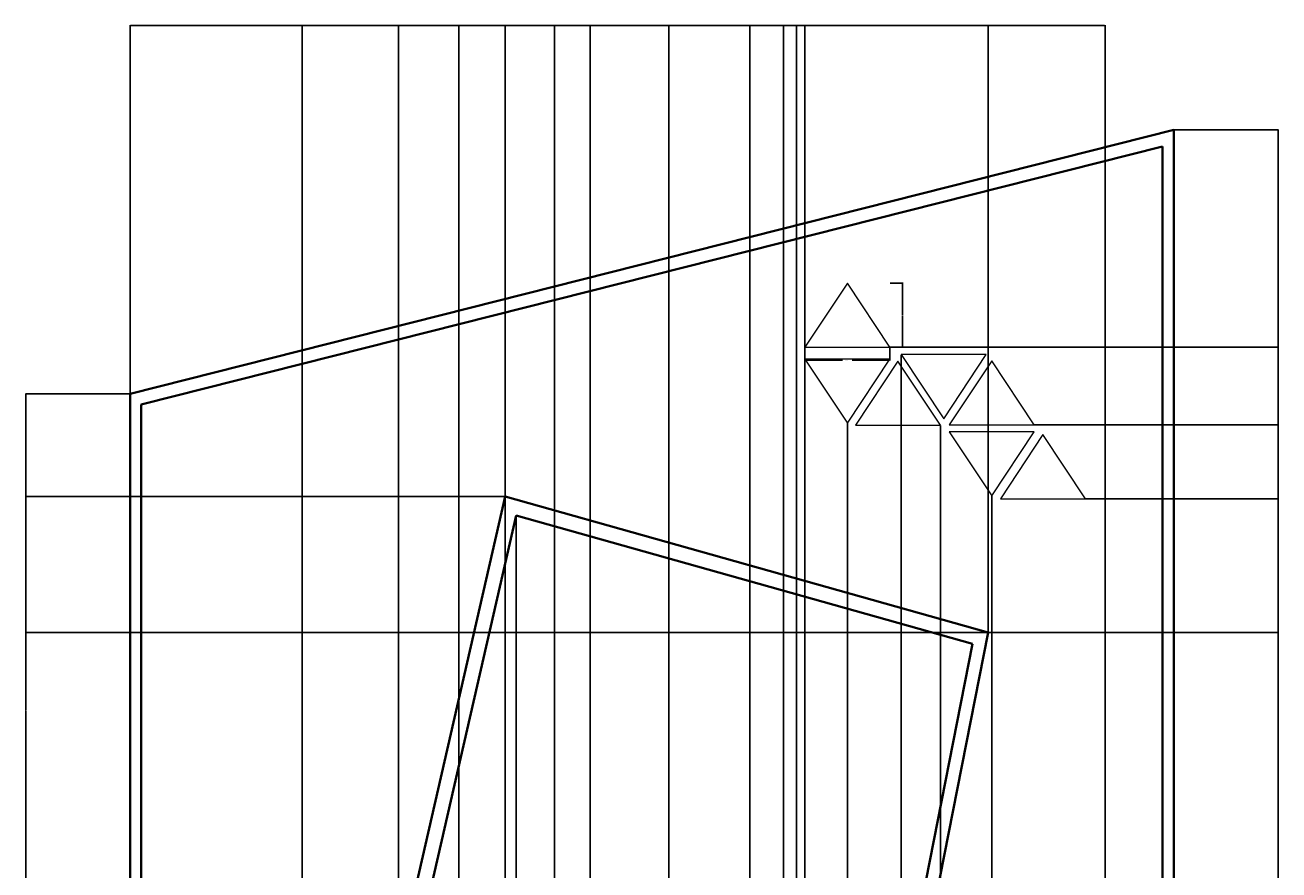
# Model space of a CAD drawing. Units: feet. Extents: x 2373 to 3800, y 799 to 1842.
# Tile 4 of 4: x 3224 to 3800, y 1453 to 1842. Entities that reach past the tile are written whole.
import ezdxf

# ---------------------------------------------------------------- set-up
doc = ezdxf.new("R2010")
doc.units = ezdxf.units.FT
for name, color, linetype, lineweight in [('A-ANNO-DIMS', 2, 'Continuous', 18), ('A-ELEV', 7, 'Continuous', 35), ('E-LITE', 2, 'Continuous', 18)]:
    doc.layers.add(name, color=color, linetype=linetype, lineweight=lineweight)
doc.styles.get("Standard").update_dxf_attribs({"font": 'arial.ttf'})
doc.dimstyles.get("Standard").update_dxf_attribs({"dimtxt": 0.18, "dimasz": 0.18, "dimexe": 0.18, "dimexo": 0.0625, "dimgap": 0.09, "dimtad": 0, "dimtih": 1, "dimtoh": 1, "dimdec": 1, "dimzin": 0, "dimdsep": 46, "dimlunit": 3, "dimtxsty": 'Standard', "dimcen": 0.09, "dimadec": 0, "dimazin": 0, "dimtfac": 1, "dimtdec": 1, "dimtofl": 0, "dimtmove": 0, "dimatfit": 3, "dimfxl": 1, "dimtolj": 1, "dimtzin": 0, "dimarcsym": 0})

# ---------------------------------------------------------------- blocks, each defined once
blk = doc.blocks.new('LIGHT-TRIANGLE')
blk.add_lwpolyline([(2765.64, 1685.95), (2746.09, 1715.45), (2726.54, 1685.95)], close=True)
blk = doc.blocks.new('*D2')
at = {"layer": 'A-ANNO-DIMS', "color": 0, "lineweight": -2, "transparency": 16777216}
for p, q in [((3582.33, 1693.47), (3582.33, 1687.49)), ((3621.43, 1693.47), (3621.43, 1687.49)), ((3582.51, 1687.67), (3599.66, 1687.67)), ((3621.25, 1687.67), (3604.1, 1687.67))]:
    blk.add_line(p, q, dxfattribs=at)
at = {"layer": 'A-ANNO-DIMS', "color": 0, "transparency": 16777216}
for points in [[(3582.51, 1687.7), (3582.51, 1687.64), (3582.33, 1687.67)], [(3621.25, 1687.7), (3621.25, 1687.64), (3621.43, 1687.67)]]:
    blk.add_solid(points, dxfattribs=at)
at = {"layer": 'Defpoints', "color": 0, "transparency": 16777216}
for p in [(3582.33, 1693.53), (3621.43, 1693.53), (3621.43, 1687.67)]:
    blk.add_point(p, dxfattribs=at)
at = {"layer": 'A-ANNO-DIMS', "color": 0, "transparency": 16777216, "insert": (3601.88, 1687.67), "char_height": 0.18, "attachment_point": 5}
blk.add_mtext('\\A1;TRIANGLE FEATURE LIGHT 39 TYP.', dxfattribs=at)
blk = doc.blocks.new('*D3')
at = {"layer": 'A-ANNO-DIMS', "color": 0, "lineweight": -2, "transparency": 16777216}
for p, q in [((3621.5, 1723.04), (3627.48, 1723.04)), ((3627.3, 1722.86), (3627.3, 1708.47)), ((3627.3, 1693.71), (3627.3, 1708.1)), ((3621.5, 1693.53), (3627.48, 1693.53))]:
    blk.add_line(p, q, dxfattribs=at)
at = {"layer": 'A-ANNO-DIMS', "color": 0, "transparency": 16777216}
for points in [[(3627.27, 1722.86), (3627.33, 1722.86), (3627.3, 1723.04)], [(3627.27, 1693.71), (3627.33, 1693.71), (3627.3, 1693.53)]]:
    blk.add_solid(points, dxfattribs=at)
at = {"layer": 'Defpoints', "color": 0, "transparency": 16777216}
for p in [(3621.43, 1723.04), (3627.3, 1723.04), (3621.43, 1693.53)]:
    blk.add_point(p, dxfattribs=at)
at = {"layer": 'A-ANNO-DIMS', "color": 0, "transparency": 16777216, "insert": (3627.3, 1708.28), "char_height": 0.18, "attachment_point": 5}
blk.add_mtext('\\A1;30 TYP.', dxfattribs=at)
blk = doc.blocks.new('*D8')
at = {"layer": 'A-ANNO-DIMS', "color": 0, "lineweight": -2, "transparency": 16777216}
for p, q in [((3752.05, 1793.54), (3800.17, 1793.54)), ((3799.99, 1793.36), (3799.99, 1320.78)), ((3799.99, 847.83), (3799.99, 1320.41)), ((3752.05, 847.65), (3800.17, 847.65))]:
    blk.add_line(p, q, dxfattribs=at)
at = {"layer": 'A-ANNO-DIMS', "color": 0, "transparency": 16777216}
for points in [[(3799.96, 1793.36), (3800.02, 1793.36), (3799.99, 1793.54)], [(3799.96, 847.83), (3800.02, 847.83), (3799.99, 847.65)]]:
    blk.add_solid(points, dxfattribs=at)
at = {"layer": 'Defpoints', "color": 0, "transparency": 16777216}
for p in [(3751.99, 1793.54), (3799.99, 1793.54), (3751.99, 847.65)]:
    blk.add_point(p, dxfattribs=at)
at = {"layer": 'A-ANNO-DIMS', "color": 0, "transparency": 16777216, "insert": (3799.99, 1320.6), "char_height": 0.18, "attachment_point": 5}
blk.add_mtext('\\A1;945.9', dxfattribs=at)
blk = doc.blocks.new('*D12')
at = {"layer": 'A-ANNO-DIMS', "color": 0, "lineweight": -2, "transparency": 16777216}
for p, q in [((3271.92, 1672.17), (3223.81, 1672.17)), ((3223.99, 1671.99), (3223.99, 1526.69)), ((3223.99, 1381.03), (3223.99, 1526.33)), ((3271.92, 1380.85), (3223.81, 1380.85))]:
    blk.add_line(p, q, dxfattribs=at)
at = {"layer": 'A-ANNO-DIMS', "color": 0, "transparency": 16777216}
for points in [[(3223.96, 1671.99), (3224.02, 1671.99), (3223.99, 1672.17)], [(3223.96, 1381.03), (3224.02, 1381.03), (3223.99, 1380.85)]]:
    blk.add_solid(points, dxfattribs=at)
at = {"layer": 'Defpoints', "color": 0, "transparency": 16777216}
for p in [(3223.99, 1672.17), (3271.99, 1672.17), (3271.99, 1380.85)]:
    blk.add_point(p, dxfattribs=at)
at = {"layer": 'A-ANNO-DIMS', "color": 0, "transparency": 16777216, "insert": (3223.99, 1526.51), "char_height": 0.18, "attachment_point": 5}
blk.add_mtext('\\A1;291.3', dxfattribs=at)
blk = doc.blocks.new('*D13')
at = {"layer": 'A-ANNO-DIMS', "color": 0, "lineweight": -2, "transparency": 16777216}
for p, q in [((3271.99, 1380.91), (3271.99, 1841.72)), ((3272.17, 1841.54), (3347.21, 1841.54)), ((3423.01, 1841.54), (3347.97, 1841.54)), ((3423.19, 1380.91), (3423.19, 1841.72))]:
    blk.add_line(p, q, dxfattribs=at)
at = {"layer": 'A-ANNO-DIMS', "color": 0, "transparency": 16777216}
for points in [[(3272.17, 1841.57), (3272.17, 1841.51), (3271.99, 1841.54)], [(3423.01, 1841.57), (3423.01, 1841.51), (3423.19, 1841.54)]]:
    blk.add_solid(points, dxfattribs=at)
at = {"layer": 'Defpoints', "color": 0, "transparency": 16777216}
for p in [(3423.19, 1841.54), (3271.99, 1380.85), (3423.19, 1380.85)]:
    blk.add_point(p, dxfattribs=at)
at = {"layer": 'A-ANNO-DIMS', "color": 0, "transparency": 16777216, "insert": (3347.59, 1841.54), "char_height": 0.18, "attachment_point": 5}
blk.add_mtext('\\A1;151.2', dxfattribs=at)
blk = doc.blocks.new('*D14')
at = {"layer": 'A-ANNO-DIMS', "color": 0, "lineweight": -2, "transparency": 16777216}
for p, q in [((3423.19, 1145.85), (3423.19, 1841.72)), ((3423.37, 1841.54), (3471.07, 1841.54)), ((3519.56, 1841.54), (3471.86, 1841.54)), ((3519.74, 1442.83), (3519.74, 1841.72))]:
    blk.add_line(p, q, dxfattribs=at)
at = {"layer": 'A-ANNO-DIMS', "color": 0, "transparency": 16777216}
for points in [[(3423.37, 1841.57), (3423.37, 1841.51), (3423.19, 1841.54)], [(3519.56, 1841.57), (3519.56, 1841.51), (3519.74, 1841.54)]]:
    blk.add_solid(points, dxfattribs=at)
at = {"layer": 'Defpoints', "color": 0, "transparency": 16777216}
for p in [(3519.74, 1841.54), (3519.74, 1442.77), (3423.19, 1145.79)]:
    blk.add_point(p, dxfattribs=at)
at = {"layer": 'A-ANNO-DIMS', "color": 0, "transparency": 16777216, "insert": (3471.46, 1841.54), "char_height": 0.18, "attachment_point": 5}
blk.add_mtext('\\A1;96.54', dxfattribs=at)
blk = doc.blocks.new('*D16')
at = {"layer": 'A-ANNO-DIMS', "color": 0, "lineweight": -2, "transparency": 16777216}
for p, q in [((3444.52, 1624.94), (3444.52, 1841.72)), ((3444.7, 1841.54), (3555.12, 1841.54)), ((3666.48, 1841.54), (3556.05, 1841.54)), ((3666.66, 1562.48), (3666.66, 1841.72))]:
    blk.add_line(p, q, dxfattribs=at)
at = {"layer": 'A-ANNO-DIMS', "color": 0, "transparency": 16777216}
for points in [[(3444.7, 1841.57), (3444.7, 1841.51), (3444.52, 1841.54)], [(3666.48, 1841.57), (3666.48, 1841.51), (3666.66, 1841.54)]]:
    blk.add_solid(points, dxfattribs=at)
at = {"layer": 'Defpoints', "color": 0, "transparency": 16777216}
for p in [(3666.66, 1841.54), (3444.52, 1624.88), (3666.66, 1562.42)]:
    blk.add_point(p, dxfattribs=at)
at = {"layer": 'A-ANNO-DIMS', "color": 0, "transparency": 16777216, "insert": (3555.59, 1841.54), "char_height": 0.18, "attachment_point": 5}
blk.add_mtext('\\A1;222.14', dxfattribs=at)
blk = doc.blocks.new('*D17')
at = {"layer": 'A-ANNO-DIMS', "color": 0, "lineweight": -2, "transparency": 16777216}
for p, q in [((3666.72, 1562.42), (3800.17, 1562.42)), ((3799.99, 1562.24), (3799.99, 1354.28)), ((3799.99, 1145.97), (3799.99, 1353.92)), ((3578.6, 1145.79), (3800.17, 1145.79))]:
    blk.add_line(p, q, dxfattribs=at)
at = {"layer": 'A-ANNO-DIMS', "color": 0, "transparency": 16777216}
for points in [[(3799.96, 1562.24), (3800.02, 1562.24), (3799.99, 1562.42)], [(3799.96, 1145.97), (3800.02, 1145.97), (3799.99, 1145.79)]]:
    blk.add_solid(points, dxfattribs=at)
at = {"layer": 'Defpoints', "color": 0, "transparency": 16777216}
for p in [(3666.66, 1562.42), (3799.99, 1562.42), (3578.54, 1145.79)]:
    blk.add_point(p, dxfattribs=at)
at = {"layer": 'A-ANNO-DIMS', "color": 0, "transparency": 16777216, "insert": (3799.99, 1354.1), "char_height": 0.18, "attachment_point": 5}
blk.add_mtext('\\A1;416.6', dxfattribs=at)
blk = doc.blocks.new('*D20')
at = {"layer": 'A-ANNO-DIMS', "color": 0, "lineweight": -2, "transparency": 16777216}
for p, q in [((3572.43, 945.53), (3572.43, 1841.72)), ((3572.61, 1841.54), (3645.95, 1841.54)), ((3720.2, 1841.54), (3646.87, 1841.54)), ((3720.38, 1113.42), (3720.38, 1841.72))]:
    blk.add_line(p, q, dxfattribs=at)
at = {"layer": 'A-ANNO-DIMS', "color": 0, "transparency": 16777216}
for points in [[(3572.61, 1841.57), (3572.61, 1841.51), (3572.43, 1841.54)], [(3720.2, 1841.57), (3720.2, 1841.51), (3720.38, 1841.54)]]:
    blk.add_solid(points, dxfattribs=at)
at = {"layer": 'Defpoints', "color": 0, "transparency": 16777216}
for p in [(3720.38, 1841.54), (3720.38, 1113.36), (3572.43, 945.46)]:
    blk.add_point(p, dxfattribs=at)
at = {"layer": 'A-ANNO-DIMS', "color": 0, "transparency": 16777216, "insert": (3646.41, 1841.54), "char_height": 0.18, "attachment_point": 5}
blk.add_mtext('\\A1;147.95', dxfattribs=at)
blk = doc.blocks.new('*D23')
at = {"layer": 'A-ANNO-DIMS', "color": 0, "lineweight": -2, "transparency": 16777216}
for p, q in [((3483.65, 925.75), (3483.65, 1841.72)), ((3483.83, 1841.54), (3519.95, 1841.54)), ((3556.84, 1841.54), (3520.73, 1841.54)), ((3557.02, 1097.65), (3557.02, 1841.72))]:
    blk.add_line(p, q, dxfattribs=at)
at = {"layer": 'A-ANNO-DIMS', "color": 0, "transparency": 16777216}
for points in [[(3483.83, 1841.57), (3483.83, 1841.51), (3483.65, 1841.54)], [(3556.84, 1841.57), (3556.84, 1841.51), (3557.02, 1841.54)]]:
    blk.add_solid(points, dxfattribs=at)
at = {"layer": 'Defpoints', "color": 0, "transparency": 16777216}
for p in [(3557.02, 1841.54), (3557.02, 1097.59), (3483.65, 925.69)]:
    blk.add_point(p, dxfattribs=at)
at = {"layer": 'A-ANNO-DIMS', "color": 0, "transparency": 16777216, "insert": (3520.34, 1841.54), "char_height": 0.18, "attachment_point": 5}
blk.add_mtext('\\A1;73.37', dxfattribs=at)
blk = doc.blocks.new('*D25')
at = {"layer": 'A-ANNO-DIMS', "color": 0, "lineweight": -2, "transparency": 16777216}
for p, q in [((3271.99, 1672.23), (3271.99, 1841.72)), ((3272.17, 1841.54), (3357.8, 1841.54)), ((3444.34, 1841.54), (3358.71, 1841.54)), ((3444.52, 1624.94), (3444.52, 1841.72))]:
    blk.add_line(p, q, dxfattribs=at)
at = {"layer": 'A-ANNO-DIMS', "color": 0, "transparency": 16777216}
for points in [[(3272.17, 1841.57), (3272.17, 1841.51), (3271.99, 1841.54)], [(3444.34, 1841.57), (3444.34, 1841.51), (3444.52, 1841.54)]]:
    blk.add_solid(points, dxfattribs=at)
at = {"layer": 'Defpoints', "color": 0, "transparency": 16777216}
for p in [(3444.52, 1841.54), (3271.99, 1672.17), (3444.52, 1624.88)]:
    blk.add_point(p, dxfattribs=at)
at = {"layer": 'A-ANNO-DIMS', "color": 0, "transparency": 16777216, "insert": (3358.25, 1841.54), "char_height": 0.18, "attachment_point": 5}
blk.add_mtext('\\A1;172.53', dxfattribs=at)
blk = doc.blocks.new('*D26')
at = {"layer": 'A-ANNO-DIMS', "color": 0, "lineweight": -2, "transparency": 16777216}
for p, q in [((3444.46, 1624.88), (3223.81, 1624.88)), ((3223.99, 1624.7), (3223.99, 1593.83)), ((3223.99, 1562.6), (3223.99, 1593.47)), ((3666.6, 1562.42), (3223.81, 1562.42))]:
    blk.add_line(p, q, dxfattribs=at)
at = {"layer": 'A-ANNO-DIMS', "color": 0, "transparency": 16777216}
for points in [[(3223.96, 1624.7), (3224.02, 1624.7), (3223.99, 1624.88)], [(3223.96, 1562.6), (3224.02, 1562.6), (3223.99, 1562.42)]]:
    blk.add_solid(points, dxfattribs=at)
at = {"layer": 'Defpoints', "color": 0, "transparency": 16777216}
for p in [(3444.52, 1624.88), (3223.99, 1562.42), (3666.66, 1562.42)]:
    blk.add_point(p, dxfattribs=at)
at = {"layer": 'A-ANNO-DIMS', "color": 0, "transparency": 16777216, "insert": (3223.99, 1593.65), "char_height": 0.18, "attachment_point": 5}
blk.add_mtext('\\A1;62.46', dxfattribs=at)
blk = doc.blocks.new('*D27')
at = {"layer": 'A-ANNO-DIMS', "color": 0, "lineweight": -2, "transparency": 16777216}
for p, q in [((3444.52, 1624.82), (3444.52, 799.47)), ((3449.58, 1616.05), (3449.58, 799.47)), ((3444.7, 799.65), (3446.65, 799.65)), ((3449.4, 799.65), (3447.44, 799.65))]:
    blk.add_line(p, q, dxfattribs=at)
at = {"layer": 'A-ANNO-DIMS', "color": 0, "transparency": 16777216}
for points in [[(3444.7, 799.68), (3444.7, 799.62), (3444.52, 799.65)], [(3449.4, 799.68), (3449.4, 799.62), (3449.58, 799.65)]]:
    blk.add_solid(points, dxfattribs=at)
at = {"layer": 'Defpoints', "color": 0, "transparency": 16777216}
for p in [(3444.52, 1624.88), (3449.58, 1616.11), (3449.58, 799.65)]:
    blk.add_point(p, dxfattribs=at)
at = {"layer": 'A-ANNO-DIMS', "color": 0, "transparency": 16777216, "insert": (3447.05, 799.65), "char_height": 0.18, "attachment_point": 5}
blk.add_mtext('\\A1;5.057', dxfattribs=at)
blk = doc.blocks.new('*D29')
at = {"layer": 'A-ANNO-DIMS', "color": 0, "lineweight": -2, "transparency": 16777216}
for p, q in [((3519.74, 1145.85), (3519.74, 1841.72)), ((3519.92, 1841.54), (3548.81, 1841.54)), ((3578.36, 1841.54), (3549.46, 1841.54)), ((3578.54, 1145.85), (3578.54, 1841.72))]:
    blk.add_line(p, q, dxfattribs=at)
at = {"layer": 'A-ANNO-DIMS', "color": 0, "transparency": 16777216}
for points in [[(3519.92, 1841.57), (3519.92, 1841.51), (3519.74, 1841.54)], [(3578.36, 1841.57), (3578.36, 1841.51), (3578.54, 1841.54)]]:
    blk.add_solid(points, dxfattribs=at)
at = {"layer": 'Defpoints', "color": 0, "transparency": 16777216}
for p in [(3578.54, 1841.54), (3519.74, 1145.79), (3578.54, 1145.79)]:
    blk.add_point(p, dxfattribs=at)
at = {"layer": 'A-ANNO-DIMS', "color": 0, "transparency": 16777216, "insert": (3549.14, 1841.54), "char_height": 0.18, "attachment_point": 5}
blk.add_mtext('\\A1;58.8', dxfattribs=at)
blk = doc.blocks.new('*D36')
at = {"layer": 'A-ANNO-DIMS', "color": 0, "lineweight": -2, "transparency": 16777216}
for p, q in [((3351.18, 1010.48), (3351.18, 1841.72)), ((3351.36, 1841.54), (3372.95, 1841.54)), ((3395.3, 1841.54), (3373.71, 1841.54)), ((3395.48, 1010.48), (3395.48, 1841.72))]:
    blk.add_line(p, q, dxfattribs=at)
at = {"layer": 'A-ANNO-DIMS', "color": 0, "transparency": 16777216}
for points in [[(3351.36, 1841.57), (3351.36, 1841.51), (3351.18, 1841.54)], [(3395.3, 1841.57), (3395.3, 1841.51), (3395.48, 1841.54)]]:
    blk.add_solid(points, dxfattribs=at)
at = {"layer": 'Defpoints', "color": 0, "transparency": 16777216}
for p in [(3395.48, 1841.54), (3351.18, 1010.41), (3395.48, 1010.41)]:
    blk.add_point(p, dxfattribs=at)
at = {"layer": 'A-ANNO-DIMS', "color": 0, "transparency": 16777216, "insert": (3373.33, 1841.54), "char_height": 0.18, "attachment_point": 5}
blk.add_mtext('\\A1;44.31', dxfattribs=at)
blk = doc.blocks.new('*D37')
at = {"layer": 'A-ANNO-DIMS', "color": 0, "lineweight": -2, "transparency": 16777216}
for p, q in [((3395.48, 1097.65), (3395.48, 1841.72)), ((3395.66, 1841.54), (3430.91, 1841.54)), ((3466.94, 1841.54), (3431.69, 1841.54)), ((3467.12, 1097.65), (3467.12, 1841.72))]:
    blk.add_line(p, q, dxfattribs=at)
at = {"layer": 'A-ANNO-DIMS', "color": 0, "transparency": 16777216}
for points in [[(3395.66, 1841.57), (3395.66, 1841.51), (3395.48, 1841.54)], [(3466.94, 1841.57), (3466.94, 1841.51), (3467.12, 1841.54)]]:
    blk.add_solid(points, dxfattribs=at)
at = {"layer": 'Defpoints', "color": 0, "transparency": 16777216}
for p in [(3467.12, 1841.54), (3395.48, 1097.59), (3467.12, 1097.59)]:
    blk.add_point(p, dxfattribs=at)
at = {"layer": 'A-ANNO-DIMS', "color": 0, "transparency": 16777216, "insert": (3431.3, 1841.54), "char_height": 0.18, "attachment_point": 5}
blk.add_mtext('\\A1;71.63', dxfattribs=at)
blk = doc.blocks.new('*D38')
at = {"layer": 'A-ANNO-DIMS', "color": 0, "lineweight": -2, "transparency": 16777216}
for p, q in [((3467.12, 1097.65), (3467.12, 1841.72)), ((3467.3, 1841.54), (3474.93, 1841.54)), ((3483.47, 1841.54), (3475.84, 1841.54)), ((3483.65, 1097.65), (3483.65, 1841.72))]:
    blk.add_line(p, q, dxfattribs=at)
at = {"layer": 'A-ANNO-DIMS', "color": 0, "transparency": 16777216}
for points in [[(3467.3, 1841.57), (3467.3, 1841.51), (3467.12, 1841.54)], [(3483.47, 1841.57), (3483.47, 1841.51), (3483.65, 1841.54)]]:
    blk.add_solid(points, dxfattribs=at)
at = {"layer": 'Defpoints', "color": 0, "transparency": 16777216}
for p in [(3483.65, 1841.54), (3467.12, 1097.59), (3483.65, 1097.59)]:
    blk.add_point(p, dxfattribs=at)
at = {"layer": 'A-ANNO-DIMS', "color": 0, "transparency": 16777216, "insert": (3475.39, 1841.54), "char_height": 0.18, "attachment_point": 5}
blk.add_mtext('\\A1;16.537', dxfattribs=at)
blk = doc.blocks.new('*D47')
at = {"layer": 'A-ANNO-DIMS', "color": 0, "lineweight": -2, "transparency": 16777216}
for p, q in [((3271.99, 1672.23), (3271.99, 1841.72)), ((3272.17, 1841.54), (3426.7, 1841.54)), ((3582.15, 1841.54), (3427.62, 1841.54)), ((3582.33, 1693.6), (3582.33, 1841.72))]:
    blk.add_line(p, q, dxfattribs=at)
at = {"layer": 'A-ANNO-DIMS', "color": 0, "transparency": 16777216}
for points in [[(3272.17, 1841.57), (3272.17, 1841.51), (3271.99, 1841.54)], [(3582.15, 1841.57), (3582.15, 1841.51), (3582.33, 1841.54)]]:
    blk.add_solid(points, dxfattribs=at)
at = {"layer": 'Defpoints', "color": 0, "transparency": 16777216}
for p in [(3582.33, 1841.54), (3582.33, 1693.53), (3271.99, 1672.17)]:
    blk.add_point(p, dxfattribs=at)
at = {"layer": 'A-ANNO-DIMS', "color": 0, "transparency": 16777216, "insert": (3427.16, 1841.54), "char_height": 0.18, "attachment_point": 5}
blk.add_mtext('\\A1;310.35', dxfattribs=at)
blk = doc.blocks.new('*D48')
at = {"layer": 'A-ANNO-DIMS', "color": 0, "lineweight": -2, "transparency": 16777216}
for p, q in [((3582.33, 1693.47), (3582.33, 799.47)), ((3601.88, 1658.52), (3601.88, 799.47)), ((3582.51, 799.65), (3591.72, 799.65)), ((3601.7, 799.65), (3592.49, 799.65))]:
    blk.add_line(p, q, dxfattribs=at)
at = {"layer": 'A-ANNO-DIMS', "color": 0, "transparency": 16777216}
for points in [[(3582.51, 799.68), (3582.51, 799.62), (3582.33, 799.65)], [(3601.7, 799.68), (3601.7, 799.62), (3601.88, 799.65)]]:
    blk.add_solid(points, dxfattribs=at)
at = {"layer": 'Defpoints', "color": 0, "transparency": 16777216}
for p in [(3582.33, 1693.53), (3601.88, 1658.58), (3601.88, 799.65)]:
    blk.add_point(p, dxfattribs=at)
at = {"layer": 'A-ANNO-DIMS', "color": 0, "transparency": 16777216, "insert": (3592.11, 799.65), "char_height": 0.18, "attachment_point": 5}
blk.add_mtext('\\A1;19.55', dxfattribs=at)
blk = doc.blocks.new('*D49')
at = {"layer": 'A-ANNO-DIMS', "color": 0, "lineweight": -2, "transparency": 16777216}
for p, q in [((3626.67, 1690.12), (3626.67, 799.47)), ((3601.88, 1658.52), (3601.88, 799.47)), ((3602.06, 799.65), (3613.88, 799.65)), ((3626.49, 799.65), (3614.67, 799.65))]:
    blk.add_line(p, q, dxfattribs=at)
at = {"layer": 'A-ANNO-DIMS', "color": 0, "transparency": 16777216}
for points in [[(3602.06, 799.68), (3602.06, 799.62), (3601.88, 799.65)], [(3626.49, 799.68), (3626.49, 799.62), (3626.67, 799.65)]]:
    blk.add_solid(points, dxfattribs=at)
at = {"layer": 'Defpoints', "color": 0, "transparency": 16777216}
for p in [(3626.67, 1690.18), (3601.88, 1658.58), (3626.67, 799.65)]:
    blk.add_point(p, dxfattribs=at)
at = {"layer": 'A-ANNO-DIMS', "color": 0, "transparency": 16777216, "insert": (3614.28, 799.65), "char_height": 0.18, "attachment_point": 5}
blk.add_mtext('\\A1;24.79', dxfattribs=at)
blk = doc.blocks.new('*D50')
at = {"layer": 'A-ANNO-DIMS', "color": 0, "lineweight": -2, "transparency": 16777216}
for p, q in [((3626.67, 1690.12), (3626.67, 799.47)), ((3644.71, 1657.64), (3644.71, 799.47)), ((3626.85, 799.65), (3635.31, 799.65)), ((3644.53, 799.65), (3636.08, 799.65))]:
    blk.add_line(p, q, dxfattribs=at)
at = {"layer": 'A-ANNO-DIMS', "color": 0, "transparency": 16777216}
for points in [[(3626.85, 799.68), (3626.85, 799.62), (3626.67, 799.65)], [(3644.53, 799.68), (3644.53, 799.62), (3644.71, 799.65)]]:
    blk.add_solid(points, dxfattribs=at)
at = {"layer": 'Defpoints', "color": 0, "transparency": 16777216}
for p in [(3626.67, 1690.18), (3644.71, 1657.7), (3644.71, 799.65)]:
    blk.add_point(p, dxfattribs=at)
at = {"layer": 'A-ANNO-DIMS', "color": 0, "transparency": 16777216, "insert": (3635.69, 799.65), "char_height": 0.18, "attachment_point": 5}
blk.add_mtext('\\A1;18.03', dxfattribs=at)
blk = doc.blocks.new('*D51')
at = {"layer": 'A-ANNO-DIMS', "color": 0, "lineweight": -2, "transparency": 16777216}
for p, q in [((3644.71, 1657.64), (3644.71, 799.47)), ((3668.27, 1625.1), (3668.27, 799.47)), ((3644.89, 799.65), (3656.02, 799.65)), ((3668.09, 799.65), (3656.95, 799.65))]:
    blk.add_line(p, q, dxfattribs=at)
at = {"layer": 'A-ANNO-DIMS', "color": 0, "transparency": 16777216}
for points in [[(3644.89, 799.68), (3644.89, 799.62), (3644.71, 799.65)], [(3668.09, 799.68), (3668.09, 799.62), (3668.27, 799.65)]]:
    blk.add_solid(points, dxfattribs=at)
at = {"layer": 'Defpoints', "color": 0, "transparency": 16777216}
for p in [(3644.71, 1657.7), (3668.27, 1625.17), (3668.27, 799.65)]:
    blk.add_point(p, dxfattribs=at)
at = {"layer": 'A-ANNO-DIMS', "color": 0, "transparency": 16777216, "insert": (3656.49, 799.65), "char_height": 0.18, "attachment_point": 5}
blk.add_mtext('\\A1;23.567', dxfattribs=at)
blk = doc.blocks.new('*D52')
at = {"layer": 'A-ANNO-DIMS', "color": 0, "lineweight": -2, "transparency": 16777216}
for p, q in [((3711.4, 1623.85), (3800.17, 1623.85)), ((3799.99, 1623.67), (3799.99, 1593.32)), ((3799.99, 1562.6), (3799.99, 1592.95)), ((3666.72, 1562.42), (3800.17, 1562.42))]:
    blk.add_line(p, q, dxfattribs=at)
at = {"layer": 'A-ANNO-DIMS', "color": 0, "transparency": 16777216}
for points in [[(3799.96, 1623.67), (3800.02, 1623.67), (3799.99, 1623.85)], [(3799.96, 1562.6), (3800.02, 1562.6), (3799.99, 1562.42)]]:
    blk.add_solid(points, dxfattribs=at)
at = {"layer": 'Defpoints', "color": 0, "transparency": 16777216}
for p in [(3711.33, 1623.85), (3799.99, 1623.85), (3666.66, 1562.42)]:
    blk.add_point(p, dxfattribs=at)
at = {"layer": 'A-ANNO-DIMS', "color": 0, "transparency": 16777216, "insert": (3799.99, 1593.14), "char_height": 0.18, "attachment_point": 5}
blk.add_mtext('\\A1;61.44', dxfattribs=at)
blk = doc.blocks.new('*D53')
at = {"layer": 'A-ANNO-DIMS', "color": 0, "lineweight": -2, "transparency": 16777216}
for p, q in [((3687.91, 1657.88), (3800.17, 1657.88)), ((3799.99, 1657.7), (3799.99, 1641.05)), ((3799.99, 1624.03), (3799.99, 1640.69)), ((3711.4, 1623.85), (3800.17, 1623.85))]:
    blk.add_line(p, q, dxfattribs=at)
at = {"layer": 'A-ANNO-DIMS', "color": 0, "transparency": 16777216}
for points in [[(3799.96, 1657.7), (3800.02, 1657.7), (3799.99, 1657.88)], [(3799.96, 1624.03), (3800.02, 1624.03), (3799.99, 1623.85)]]:
    blk.add_solid(points, dxfattribs=at)
at = {"layer": 'Defpoints', "color": 0, "transparency": 16777216}
for p in [(3687.85, 1657.88), (3799.99, 1657.88), (3711.33, 1623.85)]:
    blk.add_point(p, dxfattribs=at)
at = {"layer": 'A-ANNO-DIMS', "color": 0, "transparency": 16777216, "insert": (3799.99, 1640.87), "char_height": 0.18, "attachment_point": 5}
blk.add_mtext('\\A1;34.026', dxfattribs=at)
blk = doc.blocks.new('*D54')
at = {"layer": 'A-ANNO-DIMS', "color": 0, "lineweight": -2, "transparency": 16777216}
for p, q in [((3621.5, 1693.53), (3800.17, 1693.53)), ((3799.99, 1693.35), (3799.99, 1675.89)), ((3799.99, 1658.06), (3799.99, 1675.52)), ((3687.91, 1657.88), (3800.17, 1657.88))]:
    blk.add_line(p, q, dxfattribs=at)
at = {"layer": 'A-ANNO-DIMS', "color": 0, "transparency": 16777216}
for points in [[(3799.96, 1693.35), (3800.02, 1693.35), (3799.99, 1693.53)], [(3799.96, 1658.06), (3800.02, 1658.06), (3799.99, 1657.88)]]:
    blk.add_solid(points, dxfattribs=at)
at = {"layer": 'Defpoints', "color": 0, "transparency": 16777216}
for p in [(3621.43, 1693.53), (3799.99, 1693.53), (3687.85, 1657.88)]:
    blk.add_point(p, dxfattribs=at)
at = {"layer": 'A-ANNO-DIMS', "color": 0, "transparency": 16777216, "insert": (3799.99, 1675.71), "char_height": 0.18, "attachment_point": 5}
blk.add_mtext('\\A1;35.65', dxfattribs=at)

msp = doc.modelspace()

# ---------------------------------------------------------------- linework, layer by layer
at = {"layer": 'A-ELEV'}
for p, q in [((3271.9863, 1672.168), (3751.9863, 1793.536)), ((3751.9863, 847.6543), (3751.9863, 1793.536)), ((3277.1253, 1667.1821), (3746.8473, 1785.9513)), ((3746.8473, 1785.9513), (3746.8473, 1145.7869)), ((3271.9863, 847.6543), (3271.9863, 1672.168)), ((3277.1253, 1667.1821), (3277.1253, 1380.85)), ((3444.5198, 1624.879), (3388.5169, 1380.85)), ((3444.5198, 1624.879), (3666.6576, 1562.4189)), ((3449.5772, 1616.114), (3395.5857, 1380.85)), ((3449.5772, 1616.114), (3659.4686, 1557.0974)), ((3578.5393, 1145.7869), (3659.4686, 1557.0974)), ((3585.7283, 1151.1084), (3666.6576, 1562.4189))]:
    msp.add_line(p, q, dxfattribs=at)

# ---------------------------------------------------------------- block references
at = {"layer": 'E-LITE'}
for p in [(855.7958, 7.5847), (879.0694, -28.247), (922.2135, -28.0668), (945.6975, -62.093)]:
    msp.add_blockref('LIGHT-TRIANGLE', p, dxfattribs=at)
at = {"layer": 'E-LITE', "rotation": 180}
for p in [(6392.3111, 3376.1324), (6347.9708, 3374.0304), (6414.3606, 3340.618)]:
    msp.add_blockref('LIGHT-TRIANGLE', p, dxfattribs=at)

# ---------------------------------------------------------------- dimensions: what is measured, and where the dimension line sits
at = {"layer": 'A-ANNO-DIMS'}
for base, p1, p2, override, picture, middle in [((3423.1927, 1841.536), (3271.9863, 1380.85), (3423.1927, 1380.85), {"dimdec": 1, "dimlfac": 1, "dimrnd": 0, "dimzin": 0, "dimdsep": 46, "dimlunit": 2}, '*D13', (3347.5895, 1841.536)), ((3444.5198, 1841.536), (3271.9863, 1672.168), (3444.5198, 1624.879), {"dimdec": 2, "dimlfac": 1, "dimrnd": 0, "dimzin": 0, "dimdsep": 46, "dimlunit": 2}, '*D25', (3358.2531, 1841.536)), ((3582.3341, 1841.536), (3271.9863, 1672.168), (3582.3341, 1693.5326), {"dimdec": 2, "dimlfac": 1, "dimrnd": 0, "dimzin": 0, "dimdsep": 46, "dimlunit": 2}, '*D47', (3427.1602, 1841.536)), ((3395.4819, 1841.536), (3351.1757, 1010.4128), (3395.4819, 1010.4128), {"dimdec": 2, "dimlfac": 1, "dimrnd": 0, "dimzin": 0, "dimdsep": 46, "dimlunit": 2}, '*D36', (3373.3288, 1841.536)), ((3467.1168, 1841.536), (3395.4819, 1097.5868), (3467.1168, 1097.5868), {"dimdec": 2, "dimlfac": 1, "dimrnd": 0, "dimzin": 0, "dimdsep": 46, "dimlunit": 2}, '*D37', (3431.2994, 1841.536)), ((3519.7369, 1841.536), (3423.1927, 1145.7869), (3519.7369, 1442.7685), {"dimdec": 2, "dimlfac": 1, "dimrnd": 0, "dimzin": 0, "dimdsep": 46, "dimlunit": 2}, '*D14', (3471.4648, 1841.536)), ((3666.6576, 1841.536), (3444.5198, 1624.879), (3666.6576, 1562.4189), {"dimdec": 2, "dimlfac": 1, "dimrnd": 0, "dimzin": 0, "dimdsep": 46, "dimlunit": 2}, '*D16', (3555.5887, 1841.536)), ((3483.65428, 1841.53598), (3467.11683, 1097.58685), (3483.65428, 1097.58685), {"dimdec": 3, "dimlfac": 1, "dimrnd": 0, "dimzin": 0, "dimdsep": 46, "dimlunit": 2}, '*D38', (3475.38556, 1841.53598)), ((3557.0236, 1841.536), (3483.6543, 925.687), (3557.0236, 1097.5868), {"dimdec": 2, "dimlfac": 1, "dimrnd": 0, "dimzin": 0, "dimdsep": 46, "dimlunit": 2}, '*D23', (3520.339, 1841.536)), ((3578.5393, 1841.536), (3519.7369, 1145.7869), (3578.5393, 1145.7869), {"dimdec": 1, "dimlfac": 1, "dimrnd": 0, "dimzin": 0, "dimdsep": 46, "dimlunit": 2}, '*D29', (3549.1381, 1841.536)), ((3720.385, 1841.536), (3572.4337, 945.465), (3720.385, 1113.3603), {"dimdec": 2, "dimlfac": 1, "dimrnd": 0, "dimzin": 0, "dimdsep": 46, "dimlunit": 2}, '*D20', (3646.4093, 1841.536)), ((3601.8833, 799.6543), (3582.3341, 1693.5326), (3601.8833, 1658.579), {"dimdec": 2, "dimlfac": 1, "dimrnd": 0, "dimzin": 0, "dimdsep": 46, "dimlunit": 2}, '*D48', (3592.1087, 799.6543)), ((3626.6744, 799.6543), (3601.8833, 1658.579), (3626.6744, 1690.1846), {"dimdec": 2, "dimlfac": 1, "dimrnd": 0, "dimzin": 0, "dimdsep": 46, "dimlunit": 2}, '*D49', (3614.2788, 799.6543)), ((3644.7062, 799.6543), (3626.6744, 1690.1846), (3644.7062, 1657.7009), {"dimdec": 2, "dimlfac": 1, "dimrnd": 0, "dimzin": 0, "dimdsep": 46, "dimlunit": 2}, '*D50', (3635.6903, 799.6543)), ((3668.2731, 799.6543), (3644.7062, 1657.7009), (3668.2731, 1625.1666), {"dimdec": 3, "dimlfac": 1, "dimrnd": 0, "dimzin": 0, "dimdsep": 46, "dimlunit": 2}, '*D51', (3656.4896, 799.6543)), ((3449.5772, 799.6543), (3444.5198, 1624.879), (3449.5772, 1616.114), {"dimdec": 3, "dimlfac": 1, "dimrnd": 0, "dimzin": 0, "dimdsep": 46, "dimlunit": 2}, '*D27', (3447.0485, 799.6543))]:
    dim = msp.add_linear_dim(base=base, p1=p1, p2=p2, dimstyle='Standard', override=override, dxfattribs=at)
    dim.commit()
    dim.dimension.update_dxf_attribs({"geometry": picture, "text_midpoint": middle})
for base, p1, p2, override, picture, middle in [((3799.9863, 1793.536), (3751.9863, 847.6543), (3751.9863, 1793.536), {"dimdec": 1, "dimlfac": 1, "dimrnd": 0, "dimzin": 0, "dimdsep": 46, "dimlunit": 2}, '*D8', (3799.9863, 1320.5951)), ((3799.9863, 1693.5326), (3687.8503, 1657.8811), (3621.4325, 1693.5326), {"dimdec": 2, "dimlfac": 1, "dimrnd": 0, "dimzin": 0, "dimdsep": 46, "dimlunit": 2}, '*D54', (3799.9863, 1675.7068)), ((3223.9863, 1672.168), (3271.9863, 1380.85), (3271.9863, 1672.168), {"dimdec": 1, "dimlfac": 1, "dimrnd": 0, "dimzin": 0, "dimdsep": 46, "dimlunit": 2}, '*D12', (3223.9863, 1526.509)), ((3799.9863, 1657.8811), (3711.3342, 1623.8548), (3687.8503, 1657.8811), {"dimdec": 3, "dimlfac": 1, "dimrnd": 0, "dimzin": 0, "dimdsep": 46, "dimlunit": 2}, '*D53', (3799.9863, 1640.868)), ((3223.9863, 1562.4189), (3444.5198, 1624.879), (3666.6576, 1562.4189), {"dimdec": 2, "dimlfac": 1, "dimrnd": 0, "dimzin": 0, "dimdsep": 46, "dimlunit": 2}, '*D26', (3223.9863, 1593.649)), ((3799.9863, 1623.8548), (3666.6576, 1562.4189), (3711.3342, 1623.8548), {"dimdec": 2, "dimlfac": 1, "dimrnd": 0, "dimzin": 0, "dimdsep": 46, "dimlunit": 2}, '*D52', (3799.9863, 1593.1369)), ((3799.9863, 1562.4189), (3578.5393, 1145.7869), (3666.6576, 1562.4189), {"dimdec": 1, "dimlfac": 1, "dimrnd": 0, "dimzin": 0, "dimdsep": 46, "dimlunit": 2}, '*D17', (3799.9863, 1354.1029))]:
    dim = msp.add_linear_dim(base=base, p1=p1, p2=p2, angle=90, dimstyle='Standard', override=override, dxfattribs=at)
    dim.commit()
    dim.dimension.update_dxf_attribs({"geometry": picture, "text_midpoint": middle})
dim = msp.add_linear_dim(base=(3627.2973, 1723.0361), p1=(3621.4325, 1693.5326), p2=(3621.4325, 1723.0361), angle=90, text='<> TYP.', dimstyle='Standard', override={"dimdec": 0, "dimlfac": 1, "dimrnd": 0, "dimzin": 0, "dimdsep": 46, "dimlunit": 2}, dxfattribs=at)
dim.commit()
dim.dimension.update_dxf_attribs({"geometry": '*D3', "text_midpoint": (3627.2973, 1708.2843)})
dim = msp.add_linear_dim(base=(3621.4325, 1687.6678), p1=(3582.3341, 1693.5326), p2=(3621.4325, 1693.5326), text='TRIANGLE FEATURE LIGHT <> TYP.', dimstyle='Standard', override={"dimdec": 0, "dimlfac": 1, "dimrnd": 0, "dimzin": 0, "dimdsep": 46, "dimlunit": 2}, dxfattribs=at)
dim.commit()
dim.dimension.update_dxf_attribs({"geometry": '*D2', "text_midpoint": (3601.8833, 1687.6678)})

doc.saveas('drawing.dxf')
